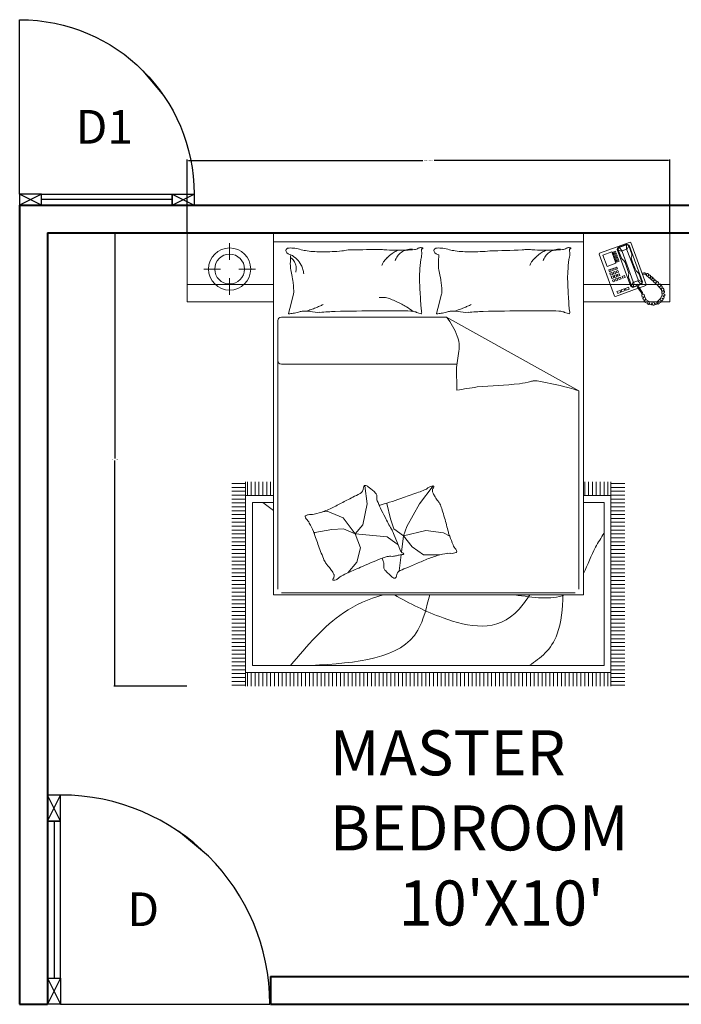
# Model space of a CAD drawing. Units: inches. Extents: x 182 to 1022, y -617 to 111.
# Tile 31 of 33: x 836 to 943, y -246 to -87. Entities that reach past the tile are written whole.
import ezdxf

# ---------------------------------------------------------------- set-up
doc = ezdxf.new("R2010")
doc.units = ezdxf.units.IN
doc.header["$MEASUREMENT"] = 0
for name, color, linetype, lineweight in [('A-ANNO-DIMS', 2, 'Continuous', 18), ('A-ANNO-IDEN', 1, 'Continuous', 18), ('A-AREA-IDEN', 8, 'Continuous', 18), ('door', 2, 'Continuous', 25), ('wall', 1, 'Continuous', 40)]:
    doc.layers.add(name, color=color, linetype=linetype, lineweight=lineweight)
doc.layers.add('furniture', color=50, linetype='Continuous', lineweight=15, transparency=0.8)
doc.styles.add('DIM_FONT', font='SIMPLEX.shx', dxfattribs={"width": 0.8})
doc.styles.get("Standard").update_dxf_attribs({"font": 'arial.ttf'})
doc.dimstyles.get("Standard").update_dxf_attribs({"dimtxt": 0.18, "dimasz": 0.18, "dimexe": 0.18, "dimexo": 0.0625, "dimgap": 0.09, "dimtad": 0, "dimtih": 1, "dimtoh": 1, "dimdec": 1, "dimzin": 0, "dimdsep": 46, "dimlunit": 4, "dimtxsty": 'Standard', "dimcen": 0.09, "dimadec": 0, "dimazin": 0, "dimtfac": 1, "dimtdec": 1, "dimtofl": 0, "dimtmove": 0, "dimatfit": 3, "dimfxl": 1, "dimtolj": 1, "dimtzin": 0, "dimarcsym": 0})

# ---------------------------------------------------------------- blocks, each defined once
blk = doc.blocks.new('A$C2D7661C6')
for p, q in [((0, 700), (50, 800)), ((50, 700), (0, 800)), ((25, 700), (25, 100)), ((50, 100), (0, 0)), ((0, 100), (50, 0))]:
    blk.add_line(p, q)
for points in [[(0, 700), (50, 700), (50, 800), (0, 800)], [(0, 100), (50, 100), (50, 700), (0, 700)], [(0, 100), (50, 100), (50, 0), (0, 0)]]:
    blk.add_lwpolyline(points, close=True)
blk.add_arc((50, 0), 800, 0, 90)
blk = doc.blocks.new('A$C7F556C88')
for p, q in [((615.7, 565.7), (500.3, 661.3)), ((50, 0), (850, 0))]:
    blk.add_line(p, q)
blk.add_blockref('A$C2D7661C6', (0, 0))
blk = doc.blocks.new('A$C4F634EDD')
for p, q in [((0, 2.6295), (0, 2.2295)), ((0.5, 2.6295), (0, 2.6295)), ((0.5, 2.6295), (2.3, 2.6295)), ((0.5, 0.5295), (0.5, 2.6295)), ((0.5, 2.2295), (0.5, 2.6295)), ((2.3, 2.6295), (2.3, 0.5295)), ((2.3, 2.6295), (2.8, 2.6295)), ((2.3, 2.2295), (2.3, 2.6295)), ((2.8, 2.6295), (2.8, 2.2295)), ((0.5, 2.5771), (2.3, 2.5771)), ((2.392, 2.5115), (2.5692, 2.5765)), ((2.5692, 2.5765), (2.574, 2.5743)), ((2.574, 2.5743), (2.6638, 2.3298)), ((0.2457, 2.5697), (0.2457, 2.4733)), ((2.412, 2.5007), (2.4634, 2.5196)), ((2.4634, 2.5196), (2.4875, 2.454)), ((2.4842, 2.5232), (2.47, 2.518)), ((2.47, 2.518), (2.472, 2.5127)), ((2.472, 2.5127), (2.4862, 2.5179)), ((2.4862, 2.5179), (2.4842, 2.5232)), ((2.4946, 2.5331), (2.4985, 2.5445)), ((2.5734, 2.3187), (2.4946, 2.5331)), ((2.4985, 2.5445), (2.5516, 2.564)), ((2.5062, 2.5454), (2.5004, 2.5392)), ((2.5004, 2.5392), (2.5013, 2.5315)), ((2.5013, 2.5315), (2.5188, 2.4836)), ((2.5013, 2.5315), (2.5231, 2.5214)), ((2.5062, 2.5454), (2.5487, 2.561)), ((2.5235, 2.5256), (2.5062, 2.5454)), ((2.5231, 2.5214), (2.5235, 2.5256)), ((2.5523, 2.4417), (2.5231, 2.5214)), ((2.5483, 2.5347), (2.5235, 2.5256)), ((2.5483, 2.5347), (2.5487, 2.561)), ((2.5514, 2.5318), (2.5483, 2.5347)), ((2.5487, 2.561), (2.5571, 2.56)), ((2.5615, 2.5536), (2.5514, 2.5318)), ((2.5807, 2.4521), (2.5514, 2.5318)), ((2.5516, 2.564), (2.5637, 2.5584)), ((2.5571, 2.56), (2.5615, 2.5536)), ((2.5615, 2.5536), (2.5791, 2.5058)), ((2.5637, 2.5584), (2.6418, 2.3458)), ((2.3898, 2.5066), (2.392, 2.5115)), ((2.4795, 2.2621), (2.3898, 2.5066)), ((2.4361, 2.4352), (2.412, 2.5007)), ((2.4881, 2.5126), (2.4739, 2.5074)), ((2.4739, 2.5074), (2.4759, 2.502)), ((2.4759, 2.502), (2.4901, 2.5073)), ((2.492, 2.5019), (2.4778, 2.4967)), ((2.4778, 2.4967), (2.4798, 2.4914)), ((2.4798, 2.4914), (2.494, 2.4966)), ((2.4959, 2.4913), (2.4817, 2.4861)), ((2.4817, 2.4861), (2.4837, 2.4808)), ((2.4837, 2.4808), (2.4979, 2.486)), ((2.4998, 2.4807), (2.4856, 2.4755)), ((2.4856, 2.4755), (2.4876, 2.4702)), ((2.4876, 2.4702), (2.5018, 2.4754)), ((2.4901, 2.5073), (2.4881, 2.5126)), ((2.5037, 2.47), (2.4895, 2.4648)), ((2.4895, 2.4648), (2.4915, 2.4595)), ((2.4915, 2.4595), (2.5057, 2.4647)), ((2.494, 2.4966), (2.492, 2.5019)), ((2.4979, 2.486), (2.4959, 2.4913)), ((2.5018, 2.4754), (2.4998, 2.4807)), ((2.5057, 2.4647), (2.5037, 2.47)), ((2.5188, 2.4836), (2.5256, 2.4761)), ((2.5256, 2.4761), (2.5342, 2.4692)), ((2.5342, 2.4692), (2.5405, 2.4574)), ((2.5405, 2.4574), (2.547, 2.4397)), ((2.5788, 2.4956), (2.5767, 2.4848)), ((2.5767, 2.4848), (2.5795, 2.4717)), ((2.5791, 2.5058), (2.5788, 2.4956)), ((2.5795, 2.4717), (2.586, 2.454)), ((0.0957, 2.4197), (0.192, 2.4197)), ((0.2994, 2.4197), (0.3957, 2.4197)), ((2.4875, 2.454), (2.4361, 2.4352)), ((2.4457, 2.4146), (2.4563, 2.4185)), ((2.4496, 2.4039), (2.4457, 2.4146)), ((2.4602, 2.4078), (2.4496, 2.4039)), ((2.4563, 2.4185), (2.4602, 2.4078)), ((2.4634, 2.4211), (2.474, 2.425)), ((2.4673, 2.4104), (2.4634, 2.4211)), ((2.4779, 2.4143), (2.4673, 2.4104)), ((2.4706, 2.4016), (2.4812, 2.4055)), ((2.4745, 2.3909), (2.4706, 2.4016)), ((2.474, 2.425), (2.4779, 2.4143)), ((2.4811, 2.4276), (2.4917, 2.4315)), ((2.485, 2.4169), (2.4811, 2.4276)), ((2.4812, 2.4055), (2.4851, 2.3949)), ((2.4956, 2.4208), (2.485, 2.4169)), ((2.4883, 2.4081), (2.4989, 2.412)), ((2.4922, 2.3975), (2.4883, 2.4081)), ((2.4917, 2.4315), (2.4956, 2.4208)), ((2.5028, 2.4014), (2.4922, 2.3975)), ((2.4989, 2.412), (2.5028, 2.4014)), ((2.5594, 2.4061), (2.547, 2.4397)), ((2.5523, 2.4417), (2.5875, 2.346)), ((2.5622, 2.393), (2.5594, 2.4061)), ((2.5807, 2.4521), (2.6158, 2.3564)), ((2.5984, 2.4204), (2.586, 2.454)), ((2.6047, 2.4086), (2.5984, 2.4204)), ((2.6133, 2.4017), (2.6047, 2.4086)), ((2.6201, 2.3941), (2.6133, 2.4017)), ((0.2457, 2.366), (0.2457, 2.2697)), ((2.4528, 2.3951), (2.4635, 2.399)), ((2.4567, 2.3844), (2.4528, 2.3951)), ((2.4674, 2.3883), (2.4567, 2.3844)), ((2.46, 2.3756), (2.4706, 2.3795)), ((2.4639, 2.365), (2.46, 2.3756)), ((2.4635, 2.399), (2.4674, 2.3883)), ((2.4745, 2.3689), (2.4639, 2.365)), ((2.4672, 2.3561), (2.4778, 2.36)), ((2.4711, 2.3455), (2.4672, 2.3561)), ((2.4706, 2.3795), (2.4745, 2.3689)), ((2.4817, 2.3494), (2.4711, 2.3455)), ((2.4851, 2.3949), (2.4745, 2.3909)), ((2.4777, 2.3821), (2.4883, 2.386)), ((2.4816, 2.3715), (2.4777, 2.3821)), ((2.4778, 2.36), (2.4817, 2.3494)), ((2.4922, 2.3754), (2.4816, 2.3715)), ((2.4849, 2.3626), (2.4955, 2.3665)), ((2.4888, 2.352), (2.4849, 2.3626)), ((2.4883, 2.386), (2.4922, 2.3754)), ((2.4994, 2.3559), (2.4888, 2.352)), ((2.4954, 2.3886), (2.5061, 2.3925)), ((2.4993, 2.378), (2.4954, 2.3886)), ((2.4955, 2.3665), (2.4994, 2.3559)), ((2.51, 2.3819), (2.4993, 2.378)), ((2.5026, 2.3691), (2.5132, 2.373)), ((2.5065, 2.3585), (2.5026, 2.3691)), ((2.5061, 2.3925), (2.51, 2.3819)), ((2.5171, 2.3624), (2.5065, 2.3585)), ((2.5132, 2.373), (2.5171, 2.3624)), ((2.5238, 2.3769), (2.538, 2.3821)), ((2.5277, 2.3663), (2.5238, 2.3769)), ((2.5419, 2.3715), (2.5277, 2.3663)), ((2.538, 2.3821), (2.5419, 2.3715)), ((2.5598, 2.372), (2.5601, 2.3822)), ((2.5774, 2.3242), (2.5598, 2.372)), ((2.5601, 2.3822), (2.5622, 2.393)), ((2.5774, 2.3242), (2.5875, 2.346)), ((2.5875, 2.346), (2.5905, 2.3431)), ((2.5905, 2.3431), (2.5901, 2.3168)), ((2.6154, 2.3522), (2.5905, 2.3431)), ((2.6158, 2.3564), (2.6154, 2.3522)), ((2.6154, 2.3522), (2.6327, 2.3324)), ((2.6376, 2.3463), (2.6158, 2.3564)), ((2.6376, 2.3463), (2.6201, 2.3941)), ((2.6418, 2.3458), (2.6369, 2.332)), ((2.6385, 2.3386), (2.6376, 2.3463)), ((2.6499, 2.3979), (2.6397, 2.3953)), ((2.6417, 2.39), (2.6488, 2.391)), ((2.6488, 2.391), (2.6538, 2.3895)), ((2.6551, 2.397), (2.6499, 2.3979)), ((2.6538, 2.3895), (2.6596, 2.388)), ((2.6627, 2.392), (2.6551, 2.397)), ((2.6596, 2.388), (2.6626, 2.3867)), ((2.6626, 2.3867), (2.6662, 2.388)), ((2.6692, 2.394), (2.6627, 2.392)), ((2.6662, 2.388), (2.6632, 2.3828)), ((2.6632, 2.3828), (2.6736, 2.3744)), ((2.6736, 2.3944), (2.6692, 2.394)), ((2.6765, 2.391), (2.6736, 2.3944)), ((2.6736, 2.3744), (2.6922, 2.3593)), ((2.6742, 2.3795), (2.6765, 2.391)), ((2.6824, 2.3858), (2.6742, 2.3795)), ((2.6873, 2.3815), (2.6824, 2.3858)), ((2.6853, 2.369), (2.6873, 2.3815)), ((2.6946, 2.376), (2.6853, 2.369)), ((2.6922, 2.3593), (2.7051, 2.3473)), ((2.6995, 2.3713), (2.6946, 2.376)), ((2.695, 2.3603), (2.6995, 2.3713)), ((2.7031, 2.3682), (2.695, 2.3603)), ((2.7096, 2.3616), (2.7031, 2.3682)), ((2.7051, 2.3473), (2.7079, 2.3475)), ((2.7062, 2.351), (2.7096, 2.3616)), ((2.7147, 2.3578), (2.7062, 2.351)), ((2.7079, 2.3475), (2.7079, 2.3443)), ((2.7079, 2.3443), (2.727, 2.3277)), ((2.7214, 2.3517), (2.7147, 2.3578)), ((2.7196, 2.34), (2.7214, 2.3517)), ((2.7286, 2.3466), (2.7196, 2.34)), ((2.7346, 2.3423), (2.7286, 2.3466)), ((2.732, 2.3295), (2.7346, 2.3423)), ((0, 2.3301), (0.5, 2.3301)), ((2.8, 2.3301), (2.3, 2.3301)), ((2.6172, 2.3086), (2.4844, 2.2599)), ((2.5114, 2.2959), (2.4936, 2.2894)), ((2.4936, 2.2894), (2.4976, 2.2788)), ((2.4976, 2.2788), (2.5153, 2.2853)), ((2.5153, 2.2853), (2.5114, 2.2959)), ((2.5362, 2.305), (2.5185, 2.2985)), ((2.5185, 2.2985), (2.5224, 2.2879)), ((2.5224, 2.2879), (2.5401, 2.2944)), ((2.5401, 2.2944), (2.5362, 2.305)), ((2.561, 2.3141), (2.5433, 2.3076)), ((2.5433, 2.3076), (2.5472, 2.297)), ((2.5472, 2.297), (2.5649, 2.3035)), ((2.5649, 2.3035), (2.561, 2.3141)), ((2.5855, 2.3131), (2.5734, 2.3187)), ((2.5818, 2.3178), (2.5774, 2.3242)), ((2.5901, 2.3168), (2.5818, 2.3178)), ((2.6104, 2.3222), (2.5855, 2.3131)), ((2.5901, 2.3168), (2.6097, 2.324)), ((2.613, 2.3312), (2.6077, 2.3293)), ((2.6077, 2.3293), (2.6135, 2.3141)), ((2.6192, 2.3174), (2.613, 2.3312)), ((2.6135, 2.3141), (2.6244, 2.2977)), ((2.6153, 2.3261), (2.6327, 2.3324)), ((2.6369, 2.332), (2.6161, 2.3243)), ((2.626, 2.3069), (2.6192, 2.3174)), ((2.6616, 2.3249), (2.6234, 2.3109)), ((2.6244, 2.2977), (2.6349, 2.2825)), ((2.6365, 2.2916), (2.626, 2.3069)), ((2.6327, 2.3324), (2.6385, 2.3386)), ((2.6407, 2.2834), (2.6365, 2.2916)), ((2.6638, 2.3298), (2.6616, 2.3249)), ((2.727, 2.3277), (2.7512, 2.2983)), ((2.7423, 2.3345), (2.732, 2.3295)), ((2.7406, 2.3172), (2.7495, 2.325)), ((2.7519, 2.3218), (2.7406, 2.3172)), ((2.7495, 2.325), (2.7423, 2.3345)), ((2.7512, 2.2983), (2.756, 2.2695)), ((2.7575, 2.3144), (2.7519, 2.3218)), ((2.7526, 2.3045), (2.7575, 2.3144)), ((2.7622, 2.308), (2.7526, 2.3045)), ((2.7574, 2.2924), (2.7673, 2.2997)), ((2.7687, 2.2905), (2.7574, 2.2924)), ((2.7673, 2.2997), (2.7622, 2.308)), ((2.7699, 2.2828), (2.7687, 2.2905)), ((0, 2.2295), (0.5, 2.2295)), ((0.5953, 2.1912), (0.616, 2.2738)), ((1.4546, 2.1912), (1.4752, 2.2738)), ((2.8, 2.2295), (2.3, 2.2295)), ((2.4844, 2.2599), (2.4795, 2.2621)), ((2.6349, 2.2825), (2.638, 2.273)), ((2.6399, 2.2712), (2.6374, 2.2659)), ((2.6374, 2.2659), (2.6398, 2.257)), ((2.638, 2.273), (2.6399, 2.2712)), ((2.6398, 2.257), (2.6509, 2.259)), ((2.6438, 2.2739), (2.6407, 2.2834)), ((2.6509, 2.259), (2.6431, 2.2492)), ((2.6431, 2.2492), (2.6473, 2.2398)), ((2.6519, 2.2716), (2.6438, 2.2739)), ((2.6473, 2.2398), (2.6592, 2.2429)), ((2.6535, 2.2628), (2.6519, 2.2716)), ((2.6592, 2.2429), (2.6521, 2.2314)), ((2.6521, 2.2314), (2.6598, 2.2248)), ((2.6636, 2.2409), (2.6535, 2.2628)), ((2.6598, 2.2248), (2.6697, 2.2309)), ((2.6836, 2.2287), (2.6636, 2.2409)), ((2.6697, 2.2309), (2.6684, 2.219)), ((2.7063, 2.2256), (2.6836, 2.2287)), ((2.7284, 2.2317), (2.7063, 2.2256)), ((2.7459, 2.2483), (2.7284, 2.2317)), ((2.7386, 2.2208), (2.7354, 2.2306)), ((2.7354, 2.2306), (2.7462, 2.2264)), ((2.756, 2.2695), (2.7459, 2.2483)), ((2.7509, 2.2314), (2.7459, 2.2418)), ((2.7459, 2.2418), (2.7568, 2.2352)), ((2.7462, 2.2264), (2.7509, 2.2314)), ((2.7529, 2.2505), (2.7645, 2.2498)), ((2.7607, 2.2424), (2.7529, 2.2505)), ((2.7568, 2.2352), (2.7607, 2.2424)), ((2.7587, 2.279), (2.7699, 2.2828)), ((2.7708, 2.2725), (2.7587, 2.279)), ((2.759, 2.2637), (2.7706, 2.2643)), ((2.7676, 2.2559), (2.759, 2.2637)), ((2.7645, 2.2498), (2.7676, 2.2559)), ((2.7706, 2.2643), (2.7708, 2.2725)), ((0.5878, 2.1612), (0.5953, 2.1912)), ((1.4471, 2.1612), (1.4546, 2.1912)), ((2.6684, 2.219), (2.6761, 2.2145)), ((2.6761, 2.2145), (2.6821, 2.2237)), ((2.6821, 2.2237), (2.6843, 2.2135)), ((2.6843, 2.2135), (2.6927, 2.2117)), ((2.6927, 2.2117), (2.6986, 2.222)), ((2.6986, 2.222), (2.7019, 2.2098)), ((2.7019, 2.2098), (2.7102, 2.2104)), ((2.7102, 2.2104), (2.7113, 2.2218)), ((2.7113, 2.2218), (2.7192, 2.2137)), ((2.7192, 2.2137), (2.7255, 2.2152)), ((2.7255, 2.2152), (2.7242, 2.2265)), ((2.7242, 2.2265), (2.7324, 2.2165)), ((2.7324, 2.2165), (2.7386, 2.2208)), ((0.5258, 2.121), (0.5258, 0.5617)), ((1.5035, 2.141), (0.5458, 2.141)), ((1.5035, 2.141), (2.2716, 1.7136)), ((1.576, 1.9433), (1.5624, 1.8479)), ((0.5458, 1.8684), (1.5653, 1.8684)), ((1.5624, 1.8479), (1.5641, 1.7178)), ((2.2716, 0.5617), (2.2716, 1.7136)), ((0.2586, 1.1753), (0.3386, 1.1753)), ((0.2586, 1.1528), (0.3386, 1.1528)), ((0.3386, 0), (0.3386, 1.1852)), ((0.3486, 1.1052), (0.3486, 1.1852)), ((0.3711, 1.1052), (0.3711, 1.1852)), ((0.3936, 1.1052), (0.3936, 1.1852)), ((0.4161, 1.1052), (0.4161, 1.1852)), ((0.4386, 1.1052), (0.4386, 1.1852)), ((0.4611, 1.1052), (0.4611, 1.1852)), ((0.4836, 1.1052), (0.4836, 1.1852)), ((1.031, 1.1612), (1.0448, 1.0581)), ((1.4276, 1.1611), (1.3484, 1.0571)), ((2.3061, 1.1052), (2.3061, 1.1852)), ((2.3286, 1.1052), (2.3286, 1.1852)), ((2.3511, 1.1052), (2.3511, 1.1852)), ((2.3736, 1.1052), (2.3736, 1.1852)), ((2.3961, 1.1052), (2.3961, 1.1852)), ((2.4186, 1.1052), (2.4186, 1.1852)), ((2.4411, 1.1052), (2.4411, 1.1852)), ((2.4588, 1.1852), (2.4588, 0)), ((2.4588, 1.1753), (2.5388, 1.1753)), ((2.4588, 1.1528), (2.5388, 1.1528)), ((0.2586, 1.1303), (0.3386, 1.1303)), ((0.2586, 1.1078), (0.3386, 1.1078)), ((0.3386, 1.1052), (0.5, 1.1052)), ((2.3, 1.1052), (2.4588, 1.1052)), ((2.4588, 1.1303), (2.5388, 1.1303)), ((2.4588, 1.1078), (2.5388, 1.1078)), ((0.2586, 1.0853), (0.3386, 1.0853)), ((0.2586, 1.0628), (0.3386, 1.0628)), ((0.2586, 1.0403), (0.3386, 1.0403)), ((0.3786, 1.0652), (0.5, 1.0652)), ((0.3786, 0.12), (0.3786, 1.0652)), ((1.0448, 1.0581), (1.019, 0.936)), ((1.1784, 0.9702), (1.1586, 1.0591)), ((1.3484, 1.0571), (1.2733, 0.9268)), ((2.3, 1.0652), (2.4188, 1.0652)), ((2.4188, 1.0652), (2.4188, 0.12)), ((2.4588, 1.0853), (2.5388, 1.0853)), ((2.4588, 1.0628), (2.5388, 1.0628)), ((2.4588, 1.0403), (2.5388, 1.0403)), ((0.2586, 1.0178), (0.3386, 1.0178)), ((0.2586, 0.9953), (0.3386, 0.9953)), ((0.2586, 0.9728), (0.3386, 0.9728)), ((0.8108, 1.0151), (0.7868, 1.0117)), ((0.9054, 0.9773), (0.8108, 1.0151)), ((0.9743, 0.8845), (0.9054, 0.9773)), ((2.4588, 1.0178), (2.5388, 1.0178)), ((2.4588, 0.9953), (2.5388, 0.9953)), ((2.4588, 0.9728), (2.5388, 0.9728)), ((0.2586, 0.9503), (0.3386, 0.9503)), ((0.2586, 0.9278), (0.3386, 0.9278)), ((1.019, 0.936), (0.9743, 0.8845)), ((1.1982, 0.9129), (1.1784, 0.9702)), ((1.2733, 0.9268), (1.2555, 0.8715)), ((2.4588, 0.9503), (2.5388, 0.9503)), ((2.4588, 0.9278), (2.5388, 0.9278)), ((0.2586, 0.9053), (0.3386, 0.9053)), ((0.2586, 0.8828), (0.3386, 0.8828)), ((0.2586, 0.8603), (0.3386, 0.8603)), ((0.7403, 0.8913), (0.737, 0.8849)), ((0.8384, 0.9085), (0.7403, 0.8913)), ((0.9072, 0.912), (0.8384, 0.9085)), ((0.9743, 0.8845), (0.9072, 0.912)), ((0.9743, 0.8845), (1.0052, 0.802)), ((0.9743, 0.8845), (1.16, 0.8656)), ((1.16, 0.8656), (1.2099, 0.8295)), ((1.1973, 0.8853), (1.2203, 0.829)), ((1.2555, 0.8715), (1.1982, 0.9129)), ((1.2555, 0.8715), (1.2437, 0.7773)), ((1.2555, 0.8715), (1.384, 0.9031)), ((1.2555, 0.8715), (1.3049, 0.8082)), ((1.384, 0.9031), (1.4868, 0.8892)), ((1.4868, 0.8892), (1.5228, 0.8692)), ((2.4588, 0.9053), (2.5388, 0.9053)), ((2.4588, 0.8828), (2.5388, 0.8828)), ((2.4588, 0.8603), (2.5388, 0.8603)), ((0.2586, 0.8378), (0.3386, 0.8378)), ((0.2586, 0.8153), (0.3386, 0.8153)), ((1.0052, 0.802), (0.9846, 0.7194)), ((1.2099, 0.8295), (1.222, 0.8209)), ((1.2203, 0.829), (1.2381, 0.7855)), ((1.3049, 0.8082), (1.3701, 0.7608)), ((2.4588, 0.8378), (2.5388, 0.8378)), ((2.4588, 0.8153), (2.5388, 0.8153)), ((0.2586, 0.7928), (0.3386, 0.7928)), ((0.2586, 0.7703), (0.3386, 0.7703)), ((0.2586, 0.7478), (0.3386, 0.7478)), ((1.2419, 0.7626), (1.23, 0.668)), ((1.3701, 0.7608), (1.463, 0.7608)), ((2.4588, 0.7928), (2.5388, 0.7928)), ((2.4588, 0.7703), (2.5388, 0.7703)), ((2.4588, 0.7478), (2.5388, 0.7478)), ((0.2586, 0.7253), (0.3386, 0.7253)), ((0.2586, 0.7028), (0.3386, 0.7028)), ((0.9846, 0.7194), (0.931, 0.6569)), ((2.4588, 0.7253), (2.5388, 0.7253)), ((2.4588, 0.7028), (2.5388, 0.7028)), ((0.2586, 0.6803), (0.3386, 0.6803)), ((0.2586, 0.6578), (0.3386, 0.6578)), ((0.2586, 0.6353), (0.3386, 0.6353)), ((2.4588, 0.6803), (2.5388, 0.6803)), ((2.4588, 0.6578), (2.5388, 0.6578)), ((2.4588, 0.6353), (2.5388, 0.6353)), ((0.2586, 0.6128), (0.3386, 0.6128)), ((0.2586, 0.5903), (0.3386, 0.5903)), ((2.4588, 0.6128), (2.5388, 0.6128)), ((2.4588, 0.5903), (2.5388, 0.5903)), ((0.2586, 0.5678), (0.3386, 0.5678)), ((0.2586, 0.5453), (0.3386, 0.5453)), ((0.2586, 0.5228), (0.3386, 0.5228)), ((2.3, 0.5295), (0.5, 0.5295)), ((0.5458, 0.5417), (2.2516, 0.5417)), ((2.4588, 0.5678), (2.5388, 0.5678)), ((2.4588, 0.5453), (2.5388, 0.5453)), ((2.4588, 0.5228), (2.5388, 0.5228)), ((0.2586, 0.5003), (0.3386, 0.5003)), ((0.2586, 0.4778), (0.3386, 0.4778)), ((2.4588, 0.5003), (2.5388, 0.5003)), ((2.4588, 0.4778), (2.5388, 0.4778)), ((0.2586, 0.4553), (0.3386, 0.4553)), ((0.2586, 0.4328), (0.3386, 0.4328)), ((0.2586, 0.4103), (0.3386, 0.4103)), ((2.4588, 0.4553), (2.5388, 0.4553)), ((2.4588, 0.4328), (2.5388, 0.4328)), ((2.4588, 0.4103), (2.5388, 0.4103)), ((0.2586, 0.3878), (0.3386, 0.3878)), ((0.2586, 0.3653), (0.3386, 0.3653)), ((0.2586, 0.3428), (0.3386, 0.3428)), ((2.4588, 0.3878), (2.5388, 0.3878)), ((2.4588, 0.3653), (2.5388, 0.3653)), ((2.4588, 0.3428), (2.5388, 0.3428)), ((0.2586, 0.3203), (0.3386, 0.3203)), ((0.2586, 0.2978), (0.3386, 0.2978)), ((2.4588, 0.3203), (2.5388, 0.3203)), ((2.4588, 0.2978), (2.5388, 0.2978)), ((0.2586, 0.2753), (0.3386, 0.2753)), ((0.2586, 0.2528), (0.3386, 0.2528)), ((0.2586, 0.2303), (0.3386, 0.2303)), ((2.4588, 0.2753), (2.5388, 0.2753)), ((2.4588, 0.2528), (2.5388, 0.2528)), ((2.4588, 0.2303), (2.5388, 0.2303)), ((0.2586, 0.2078), (0.3386, 0.2078)), ((0.2586, 0.1853), (0.3386, 0.1853)), ((2.4588, 0.2078), (2.5388, 0.2078)), ((2.4588, 0.1853), (2.5388, 0.1853)), ((0.2586, 0.1628), (0.3386, 0.1628)), ((0.2586, 0.1403), (0.3386, 0.1403)), ((0.2586, 0.1178), (0.3386, 0.1178)), ((2.4188, 0.12), (0.3786, 0.12)), ((2.4588, 0.1628), (2.5388, 0.1628)), ((2.4588, 0.1403), (2.5388, 0.1403)), ((2.4588, 0.1178), (2.5388, 0.1178)), ((0.2586, 0.0953), (0.3386, 0.0953)), ((0.2586, 0.0728), (0.3386, 0.0728)), ((2.4588, 0.08), (0.3386, 0.08)), ((0.3486, 0), (0.3486, 0.08)), ((0.3711, 0), (0.3711, 0.08)), ((0.3936, 0), (0.3936, 0.08)), ((0.4161, 0), (0.4161, 0.08)), ((0.4386, 0), (0.4386, 0.08)), ((0.4611, 0), (0.4611, 0.08)), ((0.4836, 0), (0.4836, 0.08)), ((0.5061, 0), (0.5061, 0.08)), ((0.5286, 0), (0.5286, 0.08)), ((0.5511, 0), (0.5511, 0.08)), ((0.5736, 0), (0.5736, 0.08)), ((0.5961, 0), (0.5961, 0.08)), ((0.6186, 0), (0.6186, 0.08)), ((0.6411, 0), (0.6411, 0.08)), ((0.6636, 0), (0.6636, 0.08)), ((0.6861, 0), (0.6861, 0.08)), ((0.7086, 0), (0.7086, 0.08)), ((0.7311, 0), (0.7311, 0.08)), ((0.7536, 0), (0.7536, 0.08)), ((0.7761, 0), (0.7761, 0.08)), ((0.7986, 0), (0.7986, 0.08)), ((0.8211, 0), (0.8211, 0.08)), ((0.8436, 0), (0.8436, 0.08)), ((0.8661, 0), (0.8661, 0.08)), ((0.8886, 0), (0.8886, 0.08)), ((0.9111, 0), (0.9111, 0.08)), ((0.9336, 0), (0.9336, 0.08)), ((0.9561, 0), (0.9561, 0.08)), ((0.9786, 0), (0.9786, 0.08)), ((1.0011, 0), (1.0011, 0.08)), ((1.0236, 0), (1.0236, 0.08)), ((1.0461, 0), (1.0461, 0.08)), ((1.0686, 0), (1.0686, 0.08)), ((1.0911, 0), (1.0911, 0.08)), ((1.1136, 0), (1.1136, 0.08)), ((1.1361, 0), (1.1361, 0.08)), ((1.1586, 0), (1.1586, 0.08)), ((1.1811, 0), (1.1811, 0.08)), ((1.2036, 0), (1.2036, 0.08)), ((1.2261, 0), (1.2261, 0.08)), ((1.2486, 0), (1.2486, 0.08)), ((1.2711, 0), (1.2711, 0.08)), ((1.2936, 0), (1.2936, 0.08)), ((1.3161, 0), (1.3161, 0.08)), ((1.3386, 0), (1.3386, 0.08)), ((1.3611, 0), (1.3611, 0.08)), ((1.3836, 0), (1.3836, 0.08)), ((1.4061, 0), (1.4061, 0.08)), ((1.4286, 0), (1.4286, 0.08)), ((1.4511, 0), (1.4511, 0.08)), ((1.4736, 0), (1.4736, 0.08)), ((1.4961, 0), (1.4961, 0.08)), ((1.5186, 0), (1.5186, 0.08)), ((1.5411, 0), (1.5411, 0.08)), ((1.5636, 0), (1.5636, 0.08)), ((1.5861, 0), (1.5861, 0.08)), ((1.6086, 0), (1.6086, 0.08)), ((1.6311, 0), (1.6311, 0.08)), ((1.6536, 0), (1.6536, 0.08)), ((1.6761, 0), (1.6761, 0.08)), ((1.6986, 0), (1.6986, 0.08)), ((1.7211, 0), (1.7211, 0.08)), ((1.7436, 0), (1.7436, 0.08)), ((1.7661, 0), (1.7661, 0.08)), ((1.7886, 0), (1.7886, 0.08)), ((1.8111, 0), (1.8111, 0.08)), ((1.8336, 0), (1.8336, 0.08)), ((1.8561, 0), (1.8561, 0.08)), ((1.8786, 0), (1.8786, 0.08)), ((1.9011, 0), (1.9011, 0.08)), ((1.9236, 0), (1.9236, 0.08)), ((1.9461, 0), (1.9461, 0.08)), ((1.9686, 0), (1.9686, 0.08)), ((1.9911, 0), (1.9911, 0.08)), ((2.0136, 0), (2.0136, 0.08)), ((2.0361, 0), (2.0361, 0.08)), ((2.0586, 0), (2.0586, 0.08)), ((2.0811, 0), (2.0811, 0.08)), ((2.1036, 0), (2.1036, 0.08)), ((2.1261, 0), (2.1261, 0.08)), ((2.1486, 0), (2.1486, 0.08)), ((2.1711, 0), (2.1711, 0.08)), ((2.1936, 0), (2.1936, 0.08)), ((2.2161, 0), (2.2161, 0.08)), ((2.2386, 0), (2.2386, 0.08)), ((2.2611, 0), (2.2611, 0.08)), ((2.2836, 0), (2.2836, 0.08)), ((2.3061, 0), (2.3061, 0.08)), ((2.3286, 0), (2.3286, 0.08)), ((2.3511, 0), (2.3511, 0.08)), ((2.3736, 0), (2.3736, 0.08)), ((2.3961, 0), (2.3961, 0.08)), ((2.4186, 0), (2.4186, 0.08)), ((2.4411, 0), (2.4411, 0.08)), ((2.4588, 0.0953), (2.5388, 0.0953)), ((2.4588, 0.0728), (2.5388, 0.0728)), ((0.2586, 0.0503), (0.3386, 0.0503)), ((0.2586, 0.0278), (0.3386, 0.0278)), ((0.2586, 0.0053), (0.3386, 0.0053)), ((2.4588, 0.0503), (2.5388, 0.0503)), ((2.4588, 0.0278), (2.5388, 0.0278)), ((2.4588, 0.0053), (2.5388, 0.0053))]:
    blk.add_line(p, q)
for radius in [0.1222, 0.0865]:
    blk.add_circle((0.2457, 2.4197), radius)
for centre, radius, start, end in [((0.5848, 2.5274), 0.0131, 101.2724, 206.5805), ((0.6036, 2.5368), 0.0342, 206.5805, 265.5998), ((0.5999, 2.4516), 0.0904, 90, 101.2724), ((0.5999, 2.3808), 0.1611, 81.5628, 90), ((0.5788, 2.2388), 0.3048, 74.256, 81.5628), ((0.7272, 2.7653), 0.2422, 254.256, 262.4531), ((0.7851, 3.2019), 0.6827, 262.4531, 270), ((0.7851, 3.5682), 1.049, 270, 276.0867), ((0.8402, 3.0514), 0.5293, 276.0867, 280.1899), ((1.1602, -8.1346), 10.6675, 90.30153, 91.21582), ((1.1169, 2.2433), 0.2897, 85.1982, 92.5386), ((1.2142, 3.4021), 0.8732, 265.1982, 269.4243), ((1.2362, 2.45), 0.0768, 117.2396, 128.3886), ((1.3082, 2.3102), 0.234, 110.8603, 117.2396), ((1.2204, 4.0232), 1.4943, 269.4243, 271.9079), ((1.2995, 2.4357), 0.0992, 126.0864, 143.8234), ((1.2995, 2.4357), 0.0992, 105.9352, 126.0864), ((1.2429, 3.3501), 0.8208, 271.9079, 275.2592), ((1.2995, 2.4357), 0.0992, 85.7841, 105.9352), ((1.3132, 2.5864), 0.0539, 275.2592, 300.6513), ((1.3554, 2.5152), 0.0289, 85.6975, 120.6513), ((1.3556, 2.519), 0.0251, 68.2117, 85.6975), ((1.3739, 2.5288), 0.0156, 158.0096, 201.421), ((1.3634, 2.533), 0.00428, 78.1069, 158.0096), ((1.3288, 2.5111), 0.0328, 351.8665, 21.421), ((1.3647, 2.5395), 0.00232, 258.1069, 19.564), ((1.3637, 2.5391), 0.00342, 19.564, 68.2117), ((1.444, 2.5274), 0.0131, 101.2724, 206.5805), ((1.4628, 2.5368), 0.0342, 206.5805, 265.5998), ((1.4591, 2.4516), 0.0904, 90, 101.2724), ((1.4591, 2.3808), 0.1611, 81.5628, 90), ((1.438, 2.2388), 0.3048, 74.256, 81.5628), ((1.5865, 2.7653), 0.2422, 254.256, 262.4531), ((1.6443, 3.2019), 0.6827, 262.4531, 270), ((1.6443, 3.5682), 1.049, 270, 276.0867), ((1.4785, 15.4878), 12.9656, 271.22425, 272.05324), ((1.97, 2.3805), 0.1524, 92.5386, 100.1899), ((1.9761, 2.2433), 0.2897, 85.1982, 92.5386), ((2.0734, 3.4021), 0.8732, 265.1982, 269.4243), ((2.0954, 2.45), 0.0768, 117.2396, 128.3886), ((2.1674, 2.3102), 0.234, 110.8603, 117.2396), ((2.0797, 4.0232), 1.4943, 269.4243, 271.9079), ((2.1588, 2.4357), 0.0992, 126.0864, 143.8234), ((2.1588, 2.4357), 0.0992, 105.9352, 126.0864), ((2.1021, 3.3501), 0.8208, 271.9079, 275.2592), ((2.1588, 2.4357), 0.0992, 85.7841, 105.9352), ((2.1724, 2.5864), 0.0539, 275.2592, 300.6513), ((2.2146, 2.5152), 0.0289, 85.6975, 120.6513), ((2.2149, 2.519), 0.0251, 68.2117, 85.6975), ((2.2331, 2.5288), 0.0156, 158.0096, 201.421), ((2.2226, 2.533), 0.00428, 78.1069, 158.0096), ((2.1881, 2.5111), 0.0328, 351.8665, 21.421), ((2.224, 2.5395), 0.00232, 258.1069, 19.564), ((2.2229, 2.5391), 0.00342, 19.564, 68.2117), ((1.0898, 2.4496), 0.4918, 173.7676, 180), ((0.5462, 2.4142), 0.0899, 41.4429, 53.7359), ((0.5368, 2.3783), 0.1399, 45.0976, 62.7964), ((0.5741, 2.4389), 0.0526, 25.3551, 41.4429), ((0.4851, 2.3967), 0.1511, 21.8149, 25.3551), ((0.5368, 2.3783), 0.1399, 27.3988, 45.0976), ((1.3127, 2.3625), 0.2002, 151.6832, 156.9972), ((1.1799, 2.4341), 0.0493, 140.9651, 151.6832), ((1.3165, 2.3233), 0.2252, 133.8115, 140.9651), ((1.4317, 2.2032), 0.3916, 128.3886, 133.8115), ((1.2995, 2.4357), 0.0992, 143.8234, 161.5603), ((2.2605, 2.3525), 0.9131, 172.3191, 176.6313), ((1.5522, 2.448), 0.1983, 167.8905, 172.3191), ((1.1177, 2.5413), 0.246, 347.8905, 351.8665), ((1.949, 2.4496), 0.4918, 173.7676, 180), ((2.1719, 2.3625), 0.2002, 151.6832, 156.9972), ((2.0391, 2.4341), 0.0493, 140.9651, 151.6832), ((2.1757, 2.3233), 0.2252, 133.8115, 140.9651), ((2.291, 2.2032), 0.3916, 128.3886, 133.8115), ((2.1588, 2.4357), 0.0992, 143.8234, 161.5603), ((3.1198, 2.3525), 0.9131, 172.3191, 176.6313), ((2.4114, 2.448), 0.1983, 167.8905, 172.3191), ((1.977, 2.5413), 0.246, 347.8905, 351.8665), ((0.8019, 2.4496), 0.204, 180, 189.6844), ((1.4703, 2.5637), 0.882, 189.6844, 192.1984), ((0.4345, 2.3765), 0.2056, 18.7799, 21.8149), ((0.576, 2.4246), 0.0562, 0, 18.7799), ((0.5406, 2.4246), 0.0915, 345.3149, 0), ((0.5368, 2.3783), 0.1399, 16.515, 27.3988), ((0.5368, 2.3783), 0.1399, 5.6311, 16.515), ((2.0266, 2.3663), 0.6787, 176.6313, 181.6331), ((1.6611, 2.4496), 0.204, 180, 189.6844), ((2.3295, 2.5637), 0.882, 189.6844, 192.1984), ((2.8858, 2.3663), 0.6787, 176.6313, 181.6331), ((0.2982, 2.3103), 0.3171, 8.0051, 12.1984), ((-0.0401, 2.2627), 0.6588, 2.6649, 8.0051), ((2.7128, 2.3859), 1.3652, 181.6331, 183.055), ((1.1575, 2.3103), 0.3171, 8.0051, 12.1984), ((0.8191, 2.2627), 0.6588, 2.6649, 8.0051), ((3.5721, 2.3859), 1.3652, 181.6331, 183.055), ((0.5503, 2.2902), 0.0677, 345.9548, 2.6649), ((14.9657, 3.0398), 13.6356, 183.05496, 183.50486), ((1.4096, 2.2902), 0.0677, 345.9548, 2.6649), ((15.8249, 3.0398), 13.6356, 183.05496, 183.50486), ((1.1303, 1.9835), 0.2721, 85.9172, 93.5552), ((1.1455, 2.197), 0.058, 69.3257, 85.9172), ((0.9871, 1.7772), 0.5066, 65.6735, 69.3257), ((0.6058, 0.9338), 1.4323, 63.5015, 65.6735), ((0.6807, 2.0561), 0.1197, 96.4341, 107.3864), ((0.6836, 2.0301), 0.1459, 78.4414, 96.4341), ((0.473, 2.8815), 0.7387, 287.1982, 289.428), ((0.759, 2.3985), 0.2301, 258.4414, 272.7491), ((0.473, 2.8815), 0.7387, 289.428, 291.6577), ((0.473, 2.8815), 0.7387, 291.6577, 293.4844), ((0.473, 2.8815), 0.7387, 293.4844, 295.3111), ((0.7026, 3.5718), 1.4048, 272.7491, 274.6176), ((0.9136, 0.9591), 1.2165, 92.6096, 94.6176), ((1.2501, -19.8405), 22.0183, 90.37908, 91.01965), ((1.2012, -3.5404), 5.7185, 89.7135, 90.9704), ((1.224, 1.0141), 1.164, 86.426, 89.7135), ((1.1054, 1.9358), 0.3126, 57.865, 63.5015), ((0.8841, 1.5835), 0.7286, 54.1737, 57.865), ((1.2875, 2.0302), 0.1459, 77.131, 86.426), ((1.3099, 2.1283), 0.0453, 62.7159, 77.131), ((1.6762, 2.2258), 0.3212, 183.5049, 189.9984), ((1.5399, 2.0561), 0.1197, 96.4341, 107.3864), ((1.5429, 2.0301), 0.1459, 78.4414, 96.4341), ((1.3322, 2.8815), 0.7387, 287.1982, 289.428), ((1.6182, 2.3985), 0.2301, 258.4414, 272.7491), ((1.3322, 2.8815), 0.7387, 289.428, 291.6577), ((1.3322, 2.8815), 0.7387, 291.6577, 293.4844), ((1.3322, 2.8815), 0.7387, 293.4844, 295.3111), ((1.5619, 3.5718), 1.4048, 272.7491, 274.6176), ((1.7729, 0.9591), 1.2165, 92.6096, 94.6176), ((2.1093, -19.8405), 22.0183, 90.37908, 91.01965), ((2.0605, -3.5404), 5.7185, 89.7135, 90.9704), ((2.0833, 1.0141), 1.164, 86.426, 89.7135), ((2.1467, 2.0302), 0.1459, 77.131, 86.426), ((2.1691, 2.1283), 0.0453, 62.7159, 77.131), ((2.5355, 2.2258), 0.3212, 183.5049, 189.9984), ((0.5458, 2.121), 0.02, 90, 180), ((0.5887, 2.1609), 0.000917, 165.9551, 274.0829), ((0.5695, 2.4301), 0.2708, 274.0829, 279.4841), ((0.5763, 2.3896), 0.2297, 279.4841, 287.3864), ((1.3658, 2.2367), 0.0767, 242.7159, 253.7788), ((1.3688, 2.247), 0.0875, 253.7788, 262.8796), ((1.3581, 2.1615), 0.00132, 262.8796, 343.3022), ((1.3409, 2.1667), 0.0193, 343.3022, 9.9984), ((1.448, 2.1609), 0.000917, 165.9551, 274.0829), ((1.4288, 2.4301), 0.2708, 274.0829, 279.4841), ((1.4355, 2.3896), 0.2297, 279.4841, 287.3864), ((1.2147, 1.9017), 0.3751, 20.1488, 39.6445), ((2.2251, 2.2367), 0.0767, 242.7159, 253.7788), ((2.2281, 2.247), 0.0875, 253.7788, 262.8796), ((2.2174, 2.1615), 0.00132, 262.8796, 343.3022), ((2.2001, 2.1667), 0.0193, 343.3022, 9.9984), ((1.3977, 1.9688), 0.1801, 351.8644, 20.1488), ((0.5458, 1.8884), 0.02, 180, 270), ((2.0378, 1.5789), 0.1942, 97.7304, 103.1904), ((2.0195, 1.7137), 0.0581, 79.2724, 97.7304), ((1.0582, 5.4638), 3.7801, 277.692, 279.495), ((0.6102, 18.0525), 16.3521, 273.75703, 274.62393), ((1.4194, 4.2174), 2.5158, 281.6741, 283.1904), ((1.2737, -2.2227), 4.0646, 77.0745, 79.2724), ((2.0359, 1.0981), 0.6574, 74.0648, 77.0745), ((1.7125, -0.0344), 1.8351, 72.2636, 74.0648), ((0.9863, 1.1494), 0.0359, 297.2902, 3.2455), ((1.0348, 1.1521), 0.0127, 51.1864, 183.2455), ((0.9991, 1.1077), 0.0697, 45.8726, 51.1864), ((1.0791, 1.1902), 0.0452, 225.8726, 232.4713), ((1.2846, 1.4577), 0.3825, 232.4713, 233.7837), ((0.6683, 0.6162), 0.6605, 52.7849, 53.7837), ((1.3469, 1.2115), 0.0792, 292.7069, 308.5854), ((1.4338, 1.1026), 0.0601, 110.3452, 128.5854), ((1.4251, 1.1259), 0.0352, 86.0516, 110.3452), ((1.4376, 1.1398), 0.0142, 126.5792, 169.5926), ((1.4273, 1.1567), 0.00443, 13.2808, 86.0516), ((1.4254, 1.1562), 0.0063, 306.5792, 13.2808), ((1.8575, -0.7096), 2.0162, 116.4147, 117.4999), ((-0.4173, 3.8699), 3.0972, 296.4147, 297.2902), ((0.9362, 0.9689), 0.2176, 46.4776, 52.7849), ((1.0327, 1.0706), 0.0774, 35.8936, 46.4776), ((1.0771, 1.1027), 0.0226, 351.9508, 35.8936), ((1.1449, 1.0931), 0.0458, 171.9508, 202.4162), ((0.2266, 4.0657), 3.145, 286.6085, 289.0836), ((-0.4107, 5.9078), 5.0942, 289.0836, 290.1287), ((1.0543, 1.9106), 0.8371, 290.1287, 292.7069), ((1.4996, 1.1284), 0.0771, 169.5926, 177.2714), ((1.4378, 1.1314), 0.0153, 177.2714, 194.5709), ((1.4611, 1.1374), 0.0393, 194.5709, 206.8179), ((1.7401, 1.2785), 0.352, 206.8179, 210.9056), ((1.6045, 1.1973), 0.194, 210.9056, 219.7005), ((0.5736, 1.5979), 0.6236, 290.7486, 297.4921), ((-1.8336, 6.2238), 5.8383, 297.49208, 297.84822), ((3.744, -4.3336), 6.1019, 117.49986, 117.84822), ((2.032, 1.4591), 1.0054, 202.4162, 205.0529), ((1.0922, 1.1636), 0.1166, 280.7366, 286.6085), ((2.6493, 1.7476), 1.6868, 205.0529, 207.0884), ((1.3929, 1.0217), 0.081, 26.0735, 39.7005), ((1.2892, 0.9709), 0.1965, 17.8396, 26.0735), ((-0.4304, 0.4175), 2.003, 15.2625, 17.8396), ((0.6894, 0.9832), 0.0058, 121.6917, 179.0386), ((0.7004, 0.983), 0.0168, 179.0386, 229.4914), ((0.7131, 0.9448), 0.0509, 103.0402, 121.6917), ((0.7152, 0.9361), 0.0599, 86.6119, 103.0402), ((0.7224, 1.0587), 0.063, 266.6119, 282.6252), ((0.6422, 1.4168), 0.43, 282.6252, 290.7486), ((2.541, 1.6922), 1.5652, 207.0884, 209.936), ((0.6405, 0.9128), 0.0755, 26.3332, 49.4914), ((-1.6775, -0.2344), 2.6619, 25.1732, 26.3332), ((-0.0881, 0.5109), 1.6481, 13.841, 15.2625), ((0.5689, 0.8213), 0.1798, 20.7081, 25.1732), ((0.2268, 0.692), 0.5454, 18.2369, 20.7081), ((2.3102, 1.3785), 1.6481, 198.2369, 199.6584), ((0.9989, 0.8042), 0.2143, 22.2355, 29.936), ((2.0418, 1.0357), 0.5454, 193.841, 196.3122), ((1.6908, 0.933), 0.1798, 196.3122, 200.7773), ((4.0115, 1.8135), 2.6619, 200.7773, 201.9373), ((2.6444, 1.4979), 2.003, 199.6584, 202.2355), ((1.6124, 0.8472), 0.0755, 201.9373, 225.0955), ((2.2689, -2.1899), 3.145, 111.0043, 113.4795), ((1.1834, 0.6373), 0.1166, 98.1216, 111.0043), ((1.1763, 0.687), 0.0663, 85.4882, 98.1216), ((1.1871, 0.8241), 0.0712, 265.4882, 277.6784), ((1.1727, 0.9313), 0.1794, 277.6784, 284.8807), ((1.2689, 0.569), 0.1955, 97.9822, 104.8807), ((1.2594, 0.7942), 0.0231, 202.2355, 252.8133), ((1.2465, 0.729), 0.034, 85.7407, 97.9822), ((1.2497, 0.772), 0.0092, 265.7407, 289.3799), ((1.2512, 0.7678), 0.00467, 289.3799, 72.8133), ((1.6266, 0.159), 0.6236, 106.3527, 113.0962), ((1.5721, 0.3449), 0.43, 98.2293, 106.3527), ((1.5195, 0.708), 0.063, 82.216, 98.2293), ((1.5362, 0.8298), 0.0599, 262.216, 278.6443), ((1.5375, 0.8209), 0.0509, 278.6443, 297.2959), ((1.5473, 0.7819), 0.0168, 354.6428, 45.0955), ((1.5582, 0.7808), 0.0058, 297.2959, 354.6428), ((0.9722, 0.8143), 0.1965, 202.2355, 210.4694), ((0.8727, 0.7557), 0.081, 210.4694, 224.0964), ((0.6752, 0.5644), 0.194, 35.3015, 44.0964), ((3.0455, -3.9778), 5.0942, 113.4795, 114.5246), ((0.1831, 0.4093), 1.0054, 18.0203, 19.3448), ((1.0957, 0.7061), 0.0458, 347.5549, 18.0203), ((1.1625, 0.6914), 0.0226, 167.5549, 211.4977), ((2.4404, -2.1823), 3.0972, 112.0188, 112.8944), ((0.5234, 2.5582), 2.0162, 292.0188, 293.104), ((-1.0798, 6.3161), 6.1019, 293.10398, 293.45234), ((3.6722, -4.6377), 5.8383, 113.0962, 113.45234), ((0.5462, 0.4731), 0.352, 31.2138, 35.3015), ((0.8372, 0.6345), 0.0142, 310.9751, 353.9885), ((0.8136, 0.6351), 0.0393, 18.9668, 31.2138), ((0.8364, 0.6429), 0.0153, 1.6673, 18.9668), ((0.7746, 0.6411), 0.0771, 353.9885, 1.6673), ((0.9332, 0.57), 0.0792, 117.1028, 132.9813), ((1.2784, -0.1047), 0.8371, 114.5246, 117.1028), ((1.2092, 0.72), 0.0774, 211.4977, 222.0817), ((1.3133, 0.814), 0.2176, 222.0817, 228.389), ((1.6074, 1.1451), 0.6605, 228.389, 229.3878), ((0.9284, 0.3533), 0.3825, 48.0754, 49.3878), ((1.1538, 0.6043), 0.0452, 41.4767, 48.0754), ((1.2399, 0.6804), 0.0697, 221.4767, 226.7905), ((1.2009, 0.6389), 0.0127, 226.7905, 358.8496), ((1.2495, 0.6379), 0.0359, 112.8944, 178.8496), ((0.8506, 0.6191), 0.0063, 130.9751, 197.6767), ((0.8488, 0.6185), 0.00443, 197.6767, 270.4475), ((0.8486, 0.6493), 0.0352, 270.4475, 294.7411), ((0.8382, 0.6719), 0.0601, 294.7411, 312.9813)]:
    blk.add_arc(centre, radius, start, end)
for points in [[(0.4393, 1.0652), (0.4595, 1.05), (0.4798, 1.0348), (0.5, 1.0195)], [(1.9003, 0.5295), (2.0065, 0.514), (2.1132, 0.4978), (2.1894, 0.5295)]]:
    blk.add_open_spline(points, degree=3)
for points, knots in [([(2.3, 0.6535), (2.3236, 0.7026), (2.3554, 0.7914), (2.4015, 0.8608), (2.4188, 0.8868)], [1893.525221, 1893.525221, 1893.525221, 1893.525221, 2051.902476, 2146.74457, 2146.74457, 2146.74457, 2146.74457]), ([(0.5992, 0.12), (0.6957, 0.2341), (0.8523, 0.4189), (1.0536, 0.5069), (1.136, 0.5295)], [0, 0, 0, 0, 432.822832, 701.445452, 701.445452, 701.445452, 701.445452]), ([(0.7187, 0.12), (0.9791, 0.1362), (1.326, 0.1577), (1.3868, 0.4574), (1.408, 0.5295)], [0, 0, 0, 0, 653.160442, 870.050857, 870.050857, 870.050857, 870.050857]), ([(1.2016, 0.5295), (1.2892, 0.479), (1.5144, 0.3684), (1.8265, 0.2994), (1.9681, 0.4992), (1.9875, 0.5295)], [936.534237, 936.534237, 936.534237, 936.534237, 1243.285375, 1683.261222, 1758.254386, 1758.254386, 1758.254386, 1758.254386]), ([(2.1796, 0.5295), (2.1798, 0.4519), (2.1548, 0.2369), (2.0487, 0.164), (1.9846, 0.12)], [2202.034493, 2202.034493, 2202.034493, 2202.034493, 2357.807635, 2594.446174, 2594.446174, 2594.446174, 2594.446174])]:
    blk.add_open_spline(points, degree=3, knots=knots)
at = {"style": 'DIM_FONT', "width": 0.8, "flags": 9}
for tag, p in [('YSIZE', (0.5, 2.6295)), ('XSIZE', (0.5, 2.6295)), ('XSIZE', (2.2985, 2.6295)), ('YSIZE', (2.2985, 2.6295))]:
    blk.add_attdef(tag, p, '', height=0.0005, dxfattribs=at)
blk = doc.blocks.new('*D20')
at = {"layer": 'A-ANNO-DIMS', "color": 0, "lineweight": -2, "transparency": 16777216}
for p, q in [((862.86, -121.8), (862.86, -110)), ((863.04, -110.18), (900.88, -110.18)), ((940.57, -110.18), (902.73, -110.18)), ((940.75, -121.8), (940.75, -110))]:
    blk.add_line(p, q, dxfattribs=at)
at = {"layer": 'A-ANNO-DIMS', "color": 0, "transparency": 16777216}
for points in [[(863.04, -110.15), (863.04, -110.21), (862.86, -110.18)], [(940.57, -110.15), (940.57, -110.21), (940.75, -110.18)]]:
    blk.add_solid(points, dxfattribs=at)
at = {"layer": 'Defpoints', "color": 0, "transparency": 16777216}
for p in [(940.75, -110.18), (862.86, -121.86), (940.75, -121.86)]:
    blk.add_point(p, dxfattribs=at)
at = {"layer": 'A-ANNO-DIMS', "color": 0, "transparency": 16777216, "insert": (901.8, -110.18), "char_height": 0.18, "attachment_point": 5}
blk.add_mtext('\\A1;BED 6\'-6" TYP.', dxfattribs=at)
blk = doc.blocks.new('*D21')
at = {"layer": 'A-ANNO-DIMS', "color": 0, "lineweight": -2, "transparency": 16777216}
for p, q in [((862.8, -121.86), (850.99, -121.86)), ((851.17, -122.04), (851.17, -158.26)), ((851.17, -194.84), (851.17, -158.62)), ((862.8, -195.02), (850.99, -195.02))]:
    blk.add_line(p, q, dxfattribs=at)
at = {"layer": 'A-ANNO-DIMS', "color": 0, "transparency": 16777216}
for points in [[(851.14, -122.04), (851.2, -122.04), (851.17, -121.86)], [(851.14, -194.84), (851.2, -194.84), (851.17, -195.02)]]:
    blk.add_solid(points, dxfattribs=at)
at = {"layer": 'Defpoints', "color": 0, "transparency": 16777216}
for p in [(851.17, -121.86), (862.86, -121.86), (862.86, -195.02)]:
    blk.add_point(p, dxfattribs=at)
at = {"layer": 'A-ANNO-DIMS', "color": 0, "transparency": 16777216, "insert": (851.17, -158.44), "char_height": 0.18, "attachment_point": 5}
blk.add_mtext('\\A1;6\'-1" TYP.', dxfattribs=at)

msp = doc.modelspace()

# ---------------------------------------------------------------- linework, layer by layer
at = {"layer": 'wall'}
for p, q in [((835.8, -117.37), (835.8, -246.37)), ((835.8, -117.37), (967.8, -117.37)), ((840.3, -121.87), (840.3, -246.37)), ((840.3, -121.87), (963.3, -121.87)), ((876.3, -241.87), (876.3, -246.37)), ((876.3, -241.87), (963.3, -241.87)), ((835.8, -246.37), (840.3, -246.37)), ((876.3, -246.37), (963.3, -246.37))]:
    msp.add_line(p, q, dxfattribs=at)

# ---------------------------------------------------------------- block references
at = {"layer": 'door', "xscale": -0.0351940229675722, "yscale": 0.0351940229675722, "zscale": 0.0351940229675722, "rotation": 270}
msp.add_blockref('A$C7F556C88', (835.8, -117.37), dxfattribs=at)
at = {"layer": 'door', "xscale": 0.042214023418219, "yscale": 0.042214023418219, "zscale": 0.042214023418219}
msp.add_blockref('A$C7F556C88', (840.3, -246.37), dxfattribs=at)
at = {"layer": 'furniture', "xscale": 27.81918712372317, "yscale": 27.81918712372317, "zscale": 27.81918712372317}
msp.add_blockref('A$C4F634EDD', (862.86, -195.02), dxfattribs=at)

# ---------------------------------------------------------------- texts
at = {"layer": 'A-ANNO-IDEN'}
for s, height, p in [('D1', 5.444, (844.85, -107.47)), ('D', 5.44, (853.2, -233.75))]:
    msp.add_text(s, height=height, dxfattribs=at).set_placement(p)
at = {"layer": 'A-AREA-IDEN', "insert": (885.85, -202.15), "char_height": 7.2703, "attachment_point": 1}
msp.add_mtext_dynamic_manual_height_columns("MASTER BEDROOM         10'X10'", width=56.2462, gutter_width=1.21, heights=[0], dxfattribs=at)

# ---------------------------------------------------------------- dimensions: what is measured, and where the dimension line sits
at = {"layer": 'A-ANNO-DIMS'}
dim = msp.add_linear_dim(base=(940.75, -110.18), p1=(862.86, -121.86), p2=(940.75, -121.86), text='BED <> TYP.', dimstyle='Standard', override={"dimdec": 1, "dimlfac": 1, "dimrnd": 0, "dimzin": 1, "dimdsep": 46, "dimlunit": 4, "dimfrac": 2}, dxfattribs=at)
dim.commit()
dim.dimension.update_dxf_attribs({"geometry": '*D20', "text_midpoint": (901.8, -110.18)})
dim = msp.add_linear_dim(base=(851.17, -121.86), p1=(862.86, -195.02), p2=(862.86, -121.86), angle=90, text='<> TYP.', dimstyle='Standard', override={"dimdec": 1, "dimlfac": 1, "dimrnd": 0, "dimzin": 1, "dimdsep": 46, "dimlunit": 4, "dimfrac": 2}, dxfattribs=at)
dim.commit()
dim.dimension.update_dxf_attribs({"geometry": '*D21', "text_midpoint": (851.17, -158.44)})

doc.saveas('drawing.dxf')
